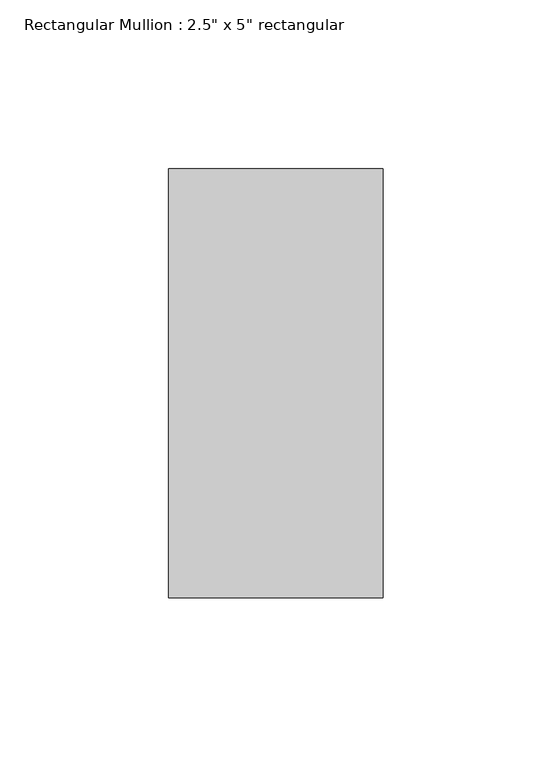
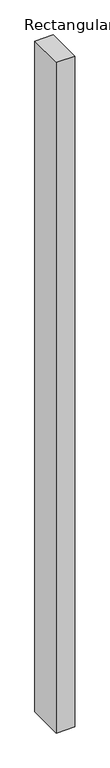
"""IFC4 building model written with IfcOpenShell, lengths in millimetres: member geometry."""

from ifc_helpers import new_model, si_unit, frame, origin, place, context, project, spatial, polyline, outline, extrude, source, transform, mapped, element, save


def member_c678549b(model_context):
    return source(origin(), model_context, "Body", "SweptSolid", [
        extrude(outline(polyline([(0.0, 63.5), (0.0, -63.5), (-63.5, -63.5), (-63.5, 63.5), (0.0, 63.5)])), frame((0.0, 0.0, -2444.75), z_axis=(0.0, 0.0, 1.0), x_axis=(1.0, 0.0, 0.0)), (0.0, 0.0, 1.0), 2444.75),
    ])


if __name__ == "__main__":
    model = new_model("IFC4")
    model_context = context("Model", 3, world=origin())
    ifc_project = project(units=[si_unit("LENGTHUNIT", "METRE", prefix="MILLI")], contexts=[model_context])
    site = spatial("IfcSite", under=ifc_project)
    building = spatial("IfcBuilding", under=site)
    placement = place(None, origin())
    member_shape = member_c678549b(model_context)
    element("IfcMember", 1, ObjectType="Rectangular Mullion : 2.5\" x 5\" rectangular", at=placement, inside=building, context=model_context, shape_type="MappedRepresentation", body=[
        mapped(member_shape, transform((0.0, 0.0, 0.0), x_axis=(1.0, 0.0, 0.0), y_axis=(0.0, 1.0, 0.0), z_axis=(0.0, 0.0, 1.0))),
    ])
    save(model, "model.ifc")

# Revit data of these elements
# Type "Rectangular Mullion : 2.5\" x 5\" rectangular"
#   built-in parameter 1007304 = 0.416667 (stored number, unit not read)
#   built-in parameter 1007301 = 0.104167 (stored number, unit not read)
#   built-in parameter 1007300 = 0.104167 (stored number, unit not read)
# Element 1 (IfcMember, "Rectangular Mullion : 2.5\" x 5\" rectangular")
#   Materials on its faces: "Aluminum"
# Materials
#   "Aluminum": class "Metal", colour RGB 247 247 247, transparency 0, Description = "Aluminum 6061", Cost = 0
